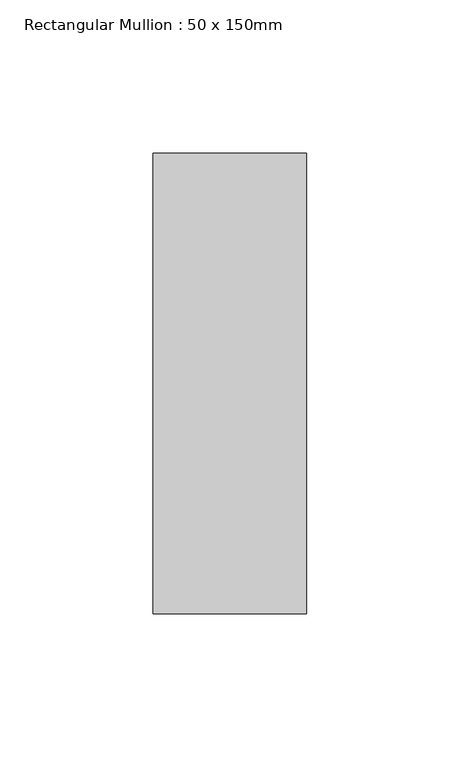
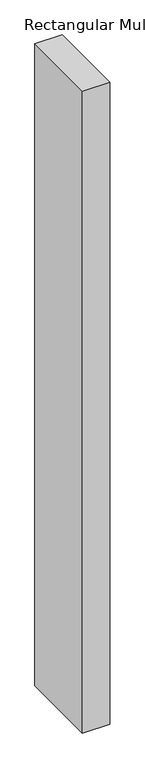
"""IFC4 building model written with IfcOpenShell, lengths in millimetres: member geometry, Rectangular Mullion : 50 x 150mm."""

from ifc_helpers import new_model, si_unit, frame, origin, place, context, project, spatial, polyline, outline, extrude, source, transform, mapped, element, save


def rectangular_mullion_50_x_150mm_bd48bb75(model_context):
    return source(origin(), model_context, "Body", "SweptSolid", [
        extrude(outline(polyline([(0.0, 75.0), (0.0, -75.0), (-50.0, -75.0), (-50.0, 75.0), (0.0, 75.0)])), frame((0.0, 0.0, -1237.4999998), z_axis=(0.0, 0.0, 1.0), x_axis=(1.0, 0.0, 0.0)), (0.0, 0.0, 1.0), 1237.4999998),
    ])


if __name__ == "__main__":
    model = new_model("IFC4")
    model_context = context("Model", 3, world=origin())
    ifc_project = project(units=[si_unit("LENGTHUNIT", "METRE", prefix="MILLI")], contexts=[model_context])
    site = spatial("IfcSite", under=ifc_project)
    building = spatial("IfcBuilding", under=site)
    placement = place(None, origin())
    rectangular_mullion_50_x_150mm_shape = rectangular_mullion_50_x_150mm_bd48bb75(model_context)
    element("IfcMember", 1, ObjectType="Rectangular Mullion : 50 x 150mm", at=placement, inside=building, context=model_context, shape_type="MappedRepresentation", body=[
        mapped(rectangular_mullion_50_x_150mm_shape, transform((0.0, 0.0, 0.0), x_axis=(1.0, 0.0, 0.0), y_axis=(0.0, 1.0, 0.0), z_axis=(0.0, 0.0, 1.0))),
    ])
    save(model, "model.ifc")

# Revit data of these elements
# Type "Rectangular Mullion : 50 x 150mm"
#   built-in parameter 1007304 = 0.492126 (stored number, unit not read)
#   built-in parameter 1007301 = 0.082021 (stored number, unit not read)
#   built-in parameter 1007300 = 0.082021 (stored number, unit not read)
# Element 1 (IfcMember, "Rectangular Mullion : 50 x 150mm")
#   Materials on its faces: "Aluminium"
# Materials
#   "Aluminium": class "Metal", colour RGB 247 247 247, transparency 0, Description = "Aluminium 6061", Cost = 0
